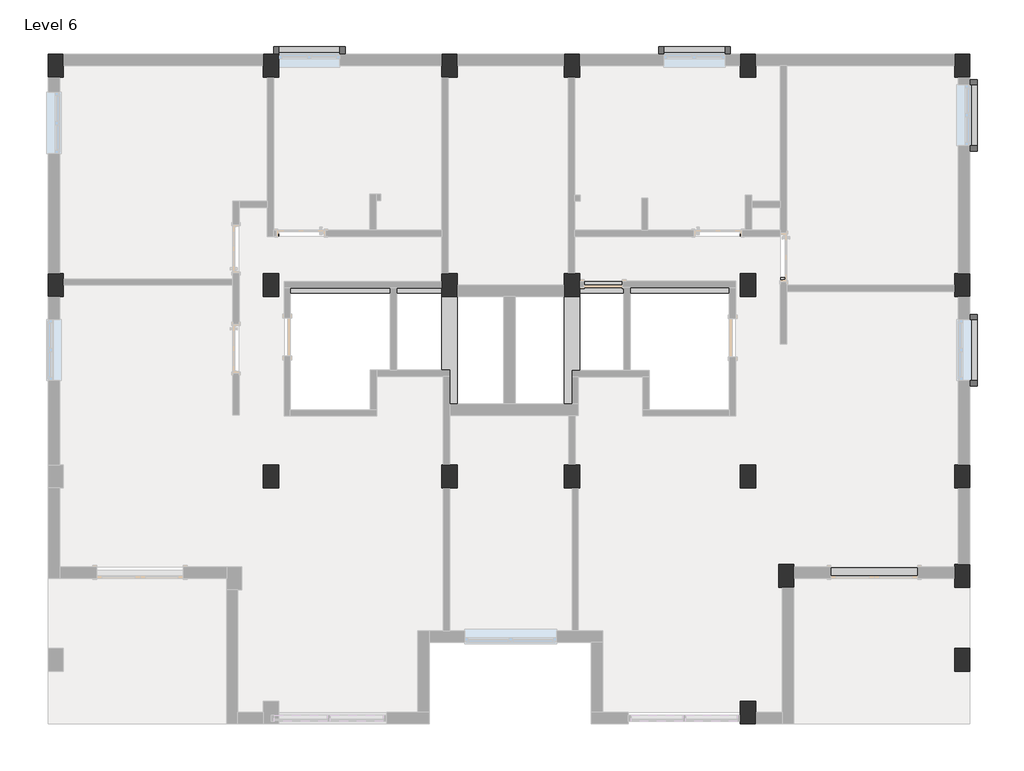
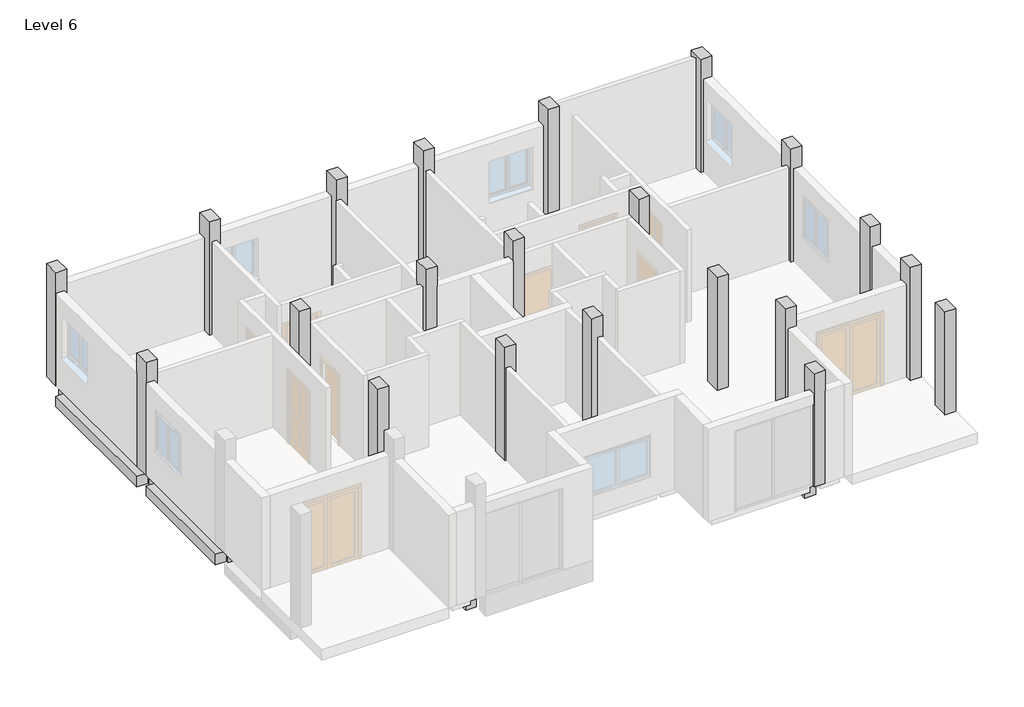
# One storey, part 3 of 3: 34 beams, 21 columns, 4 proxies.
"""IFC4 building model written with IfcOpenShell, lengths in millimetres."""

from ifc_helpers import new_model, si_unit, frame, origin, place, context, project, spatial, polyline, outline, extrude, faceted_brep, transform, mapped, element, save
from components import generic_models_13_generic_models_13_6edbfaa0, generic_models_10_generic_models_5_40bb8100, column_ab9bb308

model = new_model("IFC4")

# Units and contexts
model_context = context("Model", 3, world=origin())
ifc_project = project(units=[si_unit("LENGTHUNIT", "METRE", prefix="MILLI")], contexts=[model_context])

# Site, building, storey
site = spatial("IfcSite", under=ifc_project)
building = spatial("IfcBuilding", under=site)
storey = spatial("IfcBuildingStorey", under=building, Name="Level 6", Elevation=9448.8)

# Beams
placement = place(None, origin())
element("IfcBeam", 1, ObjectType="Concrete-Rectangular Beam : 12 x 24", at=placement, inside=storey, context=model_context, shape_type="SweptSolid", body=[
    extrude(outline(polyline([(-8839.9786397, -1604.6061634), (-8839.9786397, -1299.8061634), (-4852.9175798, -1299.8061634), (-4852.9175798, -1604.6061634), (-8839.9786397, -1604.6061634)])), frame((0.0, 0.0, 8839.2), z_axis=(0.0, 0.0, 1.0), x_axis=(1.0, 0.0, 0.0)), (0.0, 0.0, 1.0), 304.8),
])
element("IfcBeam", 2, ObjectType="Concrete-Rectangular Beam : 12 x 24", at=placement, inside=storey, context=model_context, shape_type="SweptSolid", body=[
    extrude(outline(polyline([(-1296.9175798, -1604.6061634), (-4548.1175798, -1604.6061634), (-4548.1175798, -1299.8061634), (-1296.9175798, -1299.8061634), (-1296.9175798, -1604.6061634)])), frame((0.0, 0.0, 8839.2), z_axis=(0.0, 0.0, 1.0), x_axis=(1.0, 0.0, 0.0)), (0.0, 0.0, 1.0), 304.8),
])
element("IfcBeam", 3, ObjectType="Concrete-Rectangular Beam : 12 x 24", at=placement, inside=storey, context=model_context, shape_type="SweptSolid", body=[
    extrude(outline(polyline([(1141.4824202, -1604.6061634), (-992.1175798, -1604.6061634), (-992.1175798, -1299.8061634), (1141.4824202, -1299.8061634), (1141.4824202, -1604.6061634)])), frame((0.0, 0.0, 8839.2), z_axis=(0.0, 0.0, 1.0), x_axis=(1.0, 0.0, 0.0)), (0.0, 0.0, 1.0), 304.8),
])
element("IfcBeam", 4, ObjectType="Concrete-Rectangular Beam : 12 x 24", at=placement, inside=storey, context=model_context, shape_type="SweptSolid", body=[
    extrude(outline(polyline([(4646.6824202, -1604.6061634), (1446.2824202, -1604.6061634), (1446.2824202, -1299.8061634), (4646.6824202, -1299.8061634), (4646.6824202, -1604.6061634)])), frame((0.0, 0.0, 8839.2), z_axis=(0.0, 0.0, 1.0), x_axis=(1.0, 0.0, 0.0)), (0.0, 0.0, 1.0), 304.8),
])
element("IfcBeam", 5, ObjectType="Concrete-Rectangular Beam : 12 x 24", at=placement, inside=storey, context=model_context, shape_type="SweptSolid", body=[
    extrude(outline(polyline([(8913.9345022, -1604.6061634), (4951.5345022, -1604.6061634), (4951.5345022, -1299.8061634), (8913.9345022, -1299.8061634), (8913.9345022, -1604.6061634)])), frame((0.0, 0.0, 8839.2), z_axis=(0.0, 0.0, 1.0), x_axis=(1.0, 0.0, 0.0)), (0.0, 0.0, 1.0), 304.8),
])
element("IfcBeam", 6, ObjectType="Concrete-Rectangular Beam : 12 x 24", at=placement, inside=storey, context=model_context, shape_type="SweptSolid", body=[
    extrude(outline(polyline([(8913.8824202, -5600.6620333), (8913.8824202, -1680.8061634), (9218.6824202, -1680.8061634), (9218.6824202, -5600.6620333), (8913.8824202, -5600.6620333)])), frame((0.0, 0.0, 8839.2), z_axis=(0.0, 0.0, 1.0), x_axis=(1.0, 0.0, 0.0)), (0.0, 0.0, 1.0), 304.8),
])
element("IfcBeam", 7, ObjectType="Concrete-Rectangular Beam : 12 x 24", at=placement, inside=storey, context=model_context, shape_type="SweptSolid", body=[
    extrude(outline(polyline([(8913.8824202, -9410.6620333), (8913.8824202, -6057.8620333), (9218.6824202, -6057.8620333), (9218.6824202, -9410.6620333), (8913.8824202, -9410.6620333)])), frame((0.0, 0.0, 8839.2), z_axis=(0.0, 0.0, 1.0), x_axis=(1.0, 0.0, 0.0)), (0.0, 0.0, 1.0), 304.8),
])
element("IfcBeam", 8, ObjectType="Concrete-Rectangular Beam : 12 x 24", at=placement, inside=storey, context=model_context, shape_type="SweptSolid", body=[
    extrude(outline(polyline([(8913.8824202, -11391.8620333), (8913.8824202, -9867.8620333), (9218.6824202, -9867.8620333), (9218.6824202, -11391.8620333), (8913.8824202, -11391.8620333)])), frame((0.0, 0.0, 8839.2), z_axis=(0.0, 0.0, 1.0), x_axis=(1.0, 0.0, 0.0)), (0.0, 0.0, 1.0), 304.8),
])
element("IfcBeam", 9, ObjectType="Concrete-Rectangular Beam : 12 x 24", at=placement, inside=storey, context=model_context, shape_type="SweptSolid", body=[
    extrude(outline(polyline([(-9144.7786397, -5600.6620333), (-9144.7786397, -1680.8061634), (-8839.9786397, -1680.8061634), (-8839.9786397, -5600.6620333), (-9144.7786397, -5600.6620333)])), frame((0.0, 0.0, 8839.2), z_axis=(0.0, 0.0, 1.0), x_axis=(1.0, 0.0, 0.0)), (0.0, 0.0, 1.0), 304.8),
])
element("IfcBeam", 10, ObjectType="Concrete-Rectangular Beam : 12 x 24", at=placement, inside=storey, context=model_context, shape_type="SweptSolid", body=[
    extrude(outline(polyline([(-9144.7786397, -9410.6620333), (-9144.7786397, -6057.8620333), (-8839.9786397, -6057.8620333), (-8839.9786397, -9410.6620333), (-9144.7786397, -9410.6620333)])), frame((0.0, 0.0, 8839.2), z_axis=(0.0, 0.0, 1.0), x_axis=(1.0, 0.0, 0.0)), (0.0, 0.0, 1.0), 304.8),
])
element("IfcBeam", 11, ObjectType="Concrete-Rectangular Beam : 12 x 24", at=placement, inside=storey, context=model_context, shape_type="SweptSolid", body=[
    extrude(outline(polyline([(4951.4824202, -5676.8620333), (8913.8824202, -5676.8620333), (8913.8824202, -5981.6620333), (4951.4824202, -5981.6620333), (4951.4824202, -5676.8620333)])), frame((0.0, 0.0, 8839.2), z_axis=(0.0, 0.0, 1.0), x_axis=(1.0, 0.0, 0.0)), (0.0, 0.0, 1.0), 304.8),
])
element("IfcBeam", 12, ObjectType="Concrete-Rectangular Beam : 12 x 24", at=placement, inside=storey, context=model_context, shape_type="SweptSolid", body=[
    extrude(outline(polyline([(1446.2824202, -5676.8620333), (4646.6824202, -5676.8620333), (4646.6824202, -5981.6620333), (1446.2824202, -5981.6620333), (1446.2824202, -5676.8620333)])), frame((0.0, 0.0, 8839.2), z_axis=(0.0, 0.0, 1.0), x_axis=(1.0, 0.0, 0.0)), (0.0, 0.0, 1.0), 304.8),
])
element("IfcBeam", 13, ObjectType="Concrete-Rectangular Beam : 12 x 24", at=placement, inside=storey, context=model_context, shape_type="SweptSolid", body=[
    extrude(outline(polyline([(-992.1175798, -5676.8620333), (1141.4824202, -5676.8620333), (1141.4824202, -5981.6620333), (-992.1175798, -5981.6620333), (-992.1175798, -5676.8620333)])), frame((0.0, 0.0, 8839.2), z_axis=(0.0, 0.0, 1.0), x_axis=(1.0, 0.0, 0.0)), (0.0, 0.0, 1.0), 304.8),
])
element("IfcBeam", 14, ObjectType="Concrete-Rectangular Beam : 12 x 24", at=placement, inside=storey, context=model_context, shape_type="SweptSolid", body=[
    extrude(outline(polyline([(-4548.1175798, -5676.8620333), (-1296.9175798, -5676.8620333), (-1296.9175798, -5981.6620333), (-4548.1175798, -5981.6620333), (-4548.1175798, -5676.8620333)])), frame((0.0, 0.0, 8839.2), z_axis=(0.0, 0.0, 1.0), x_axis=(1.0, 0.0, 0.0)), (0.0, 0.0, 1.0), 304.8),
])
element("IfcBeam", 15, ObjectType="Concrete-Rectangular Beam : 12 x 24", at=placement, inside=storey, context=model_context, shape_type="SweptSolid", body=[
    extrude(outline(polyline([(-8839.9786397, -5676.8620333), (-4852.9175798, -5676.8620333), (-4852.9175798, -5981.6620333), (-8839.9786397, -5981.6620333), (-8839.9786397, -5676.8620333)])), frame((0.0, 0.0, 8839.2), z_axis=(0.0, 0.0, 1.0), x_axis=(1.0, 0.0, 0.0)), (0.0, 0.0, 1.0), 304.8),
])
element("IfcBeam", 16, ObjectType="Concrete-Rectangular Beam : 12 x 24", at=placement, inside=storey, context=model_context, shape_type="SweptSolid", body=[
    extrude(outline(polyline([(-4852.9175798, -9791.6620333), (-8839.9786397, -9791.6620333), (-8839.9786397, -9486.8620333), (-4852.9175798, -9486.8620333), (-4852.9175798, -9791.6620333)])), frame((0.0, 0.0, 8839.2), z_axis=(0.0, 0.0, 1.0), x_axis=(1.0, 0.0, 0.0)), (0.0, 0.0, 1.0), 304.8),
])
element("IfcBeam", 17, ObjectType="Concrete-Rectangular Beam : 12 x 24", at=placement, inside=storey, context=model_context, shape_type="SweptSolid", body=[
    extrude(outline(polyline([(-1296.9175798, -9791.6620333), (-4548.1175798, -9791.6620333), (-4548.1175798, -9486.8620333), (-1296.9175798, -9486.8620333), (-1296.9175798, -9791.6620333)])), frame((0.0, 0.0, 8839.2), z_axis=(0.0, 0.0, 1.0), x_axis=(1.0, 0.0, 0.0)), (0.0, 0.0, 1.0), 304.8),
])
element("IfcBeam", 18, ObjectType="Concrete-Rectangular Beam : 12 x 24", at=placement, inside=storey, context=model_context, shape_type="SweptSolid", body=[
    extrude(outline(polyline([(1446.2824202, -9791.6620333), (1446.2824202, -9486.8620333), (4646.6824202, -9486.8620333), (4646.6824202, -9791.6620333), (1446.2824202, -9791.6620333)])), frame((0.0, 0.0, 8839.2), z_axis=(0.0, 0.0, 1.0), x_axis=(1.0, 0.0, 0.0)), (0.0, 0.0, 1.0), 304.8),
])
element("IfcBeam", 19, ObjectType="Concrete-Rectangular Beam : 12 x 24", at=placement, inside=storey, context=model_context, shape_type="Brep", body=[
    faceted_brep([(4646.6824202, -9867.8620333, 8839.2), (4646.6824202, -11772.8620333, 8839.2), (4646.6824202, -11772.8620333, 9144.0), (4646.6824202, -9867.8620333, 9144.0), (4951.4824202, -9867.8620333, 8839.2), (4951.4824202, -11468.0620333, 8839.2), (4951.4824202, -11772.8620333, 8839.2), (4951.4824202, -9867.8620333, 9144.0), (4951.4824202, -11468.0620333, 9144.0), (4951.4824202, -11772.8620333, 9144.0)], [[[0, 1, 2, 3]], [[1, 0, 4, 5, 6]], [[6, 5, 4, 7, 8, 9]], [[1, 6, 9, 2]], [[4, 0, 3, 7]], [[3, 2, 9, 8, 7]]]),
])
element("IfcBeam", 20, ObjectType="Concrete-Rectangular Beam : 12 x 24", at=placement, inside=storey, context=model_context, shape_type="SweptSolid", body=[
    extrude(outline(polyline([(4951.4824202, -11772.8620333), (4951.4824202, -11468.0620333), (5408.6824202, -11468.0620333), (5408.6824202, -11772.8620333), (4951.4824202, -11772.8620333)])), frame((0.0, 0.0, 8839.2), z_axis=(0.0, 0.0, 1.0), x_axis=(1.0, 0.0, 0.0)), (0.0, 0.0, 1.0), 304.8),
])
element("IfcBeam", 21, ObjectType="Concrete-Rectangular Beam : 12 x 24", at=placement, inside=storey, context=model_context, shape_type="SweptSolid", body=[
    extrude(outline(polyline([(8913.8824202, -11772.8620333), (5713.4824202, -11772.8620333), (5713.4824202, -11468.0620333), (8913.8824202, -11468.0620333), (8913.8824202, -11772.8620333)])), frame((0.0, 0.0, 8839.2), z_axis=(0.0, 0.0, 1.0), x_axis=(1.0, 0.0, 0.0)), (0.0, 0.0, 1.0), 304.8),
])
element("IfcBeam", 22, ObjectType="Concrete-Rectangular Beam : 12 x 24", at=placement, inside=storey, context=model_context, shape_type="Brep", body=[
    faceted_brep([(-4852.9175798, -9867.8620333, 8839.2), (-4852.9175798, -11518.8620333, 8839.2), (-4852.9175798, -11823.6620333, 8839.2), (-4852.9175798, -14119.6402089, 8839.2), (-4852.9175798, -14119.6402089, 9144.0), (-4852.9175798, -11823.6620333, 9144.0), (-4852.9175798, -11518.8620333, 9144.0), (-4852.9175798, -9867.8620333, 9144.0), (-4548.1175798, -9867.8620333, 8839.2), (-4548.1175798, -14119.6402089, 8839.2), (-4548.1175798, -9867.8620333, 9144.0), (-4548.1175798, -14119.6402089, 9144.0)], [[[0, 1, 2, 3, 4, 5, 6, 7]], [[3, 2, 1, 0, 8, 9]], [[9, 8, 10, 11]], [[8, 0, 7, 10]], [[3, 9, 11, 4]], [[7, 6, 5, 4, 11, 10]]]),
])
element("IfcBeam", 23, ObjectType="Concrete-Rectangular Beam : 12 x 24", at=placement, inside=storey, context=model_context, shape_type="SweptSolid", body=[
    extrude(outline(polyline([(-4852.9175798, -11823.6620333), (-5284.7175798, -11823.6620333), (-5284.7175798, -11518.8620333), (-4852.9175798, -11518.8620333), (-4852.9175798, -11823.6620333)])), frame((0.0, 0.0, 8839.2), z_axis=(0.0, 0.0, 1.0), x_axis=(1.0, 0.0, 0.0)), (0.0, 0.0, 1.0), 304.8),
])
element("IfcBeam", 24, ObjectType="Concrete-Rectangular Beam : 12 x 24", at=placement, inside=storey, context=model_context, shape_type="SweptSolid", body=[
    extrude(outline(polyline([(4951.4824202, -11772.8620333), (4951.4824202, -14119.6402089), (4646.6824202, -14119.6402089), (4646.6824202, -11772.8620333), (4951.4824202, -11772.8620333)])), frame((0.0, 0.0, 8839.2), z_axis=(0.0, 0.0, 1.0), x_axis=(1.0, 0.0, 0.0)), (0.0, 0.0, 1.0), 304.8),
])
element("IfcBeam", 25, ObjectType="Concrete-Rectangular Beam : 12 x 24", at=placement, inside=storey, context=model_context, shape_type="SweptSolid", body=[
    extrude(outline(polyline([(-4852.9175798, -5600.6620333), (-4852.9175798, -1680.8061634), (-4548.1175798, -1680.8061634), (-4548.1175798, -5600.6620333), (-4852.9175798, -5600.6620333)])), frame((0.0, 0.0, 8839.2), z_axis=(0.0, 0.0, 1.0), x_axis=(1.0, 0.0, 0.0)), (0.0, 0.0, 1.0), 304.8),
])
element("IfcBeam", 26, ObjectType="Concrete-Rectangular Beam : 12 x 24", at=placement, inside=storey, context=model_context, shape_type="SweptSolid", body=[
    extrude(outline(polyline([(-4852.9175798, -9410.6620333), (-4852.9175798, -6057.8620333), (-4548.1175798, -6057.8620333), (-4548.1175798, -9410.6620333), (-4852.9175798, -9410.6620333)])), frame((0.0, 0.0, 8839.2), z_axis=(0.0, 0.0, 1.0), x_axis=(1.0, 0.0, 0.0)), (0.0, 0.0, 1.0), 304.8),
])
element("IfcBeam", 27, ObjectType="Concrete-Rectangular Beam : 12 x 24", at=placement, inside=storey, context=model_context, shape_type="SweptSolid", body=[
    extrude(outline(polyline([(-1296.9175798, -5600.6620333), (-1296.9175798, -1680.8061634), (-992.1175798, -1680.8061634), (-992.1175798, -5600.6620333), (-1296.9175798, -5600.6620333)])), frame((0.0, 0.0, 8839.2), z_axis=(0.0, 0.0, 1.0), x_axis=(1.0, 0.0, 0.0)), (0.0, 0.0, 1.0), 304.8),
])
element("IfcBeam", 28, ObjectType="Concrete-Rectangular Beam : 12 x 24", at=placement, inside=storey, context=model_context, shape_type="SweptSolid", body=[
    extrude(outline(polyline([(-1296.9175798, -9410.6620333), (-1296.9175798, -6057.8620333), (-992.1175798, -6057.8620333), (-992.1175798, -9410.6620333), (-1296.9175798, -9410.6620333)])), frame((0.0, 0.0, 8839.2), z_axis=(0.0, 0.0, 1.0), x_axis=(1.0, 0.0, 0.0)), (0.0, 0.0, 1.0), 304.8),
])
element("IfcBeam", 29, ObjectType="Concrete-Rectangular Beam : 12 x 24", at=placement, inside=storey, context=model_context, shape_type="SweptSolid", body=[
    extrude(outline(polyline([(1446.2824202, -6057.8620333), (1446.2824202, -9410.6620333), (1141.4824202, -9410.6620333), (1141.4824202, -6057.8620333), (1446.2824202, -6057.8620333)])), frame((0.0, 0.0, 8839.2), z_axis=(0.0, 0.0, 1.0), x_axis=(1.0, 0.0, 0.0)), (0.0, 0.0, 1.0), 304.8),
])
element("IfcBeam", 30, ObjectType="Concrete-Rectangular Beam : 12 x 24", at=placement, inside=storey, context=model_context, shape_type="SweptSolid", body=[
    extrude(outline(polyline([(1446.2824202, -1680.8061634), (1446.2824202, -5600.6620333), (1141.4824202, -5600.6620333), (1141.4824202, -1680.8061634), (1446.2824202, -1680.8061634)])), frame((0.0, 0.0, 8839.2), z_axis=(0.0, 0.0, 1.0), x_axis=(1.0, 0.0, 0.0)), (0.0, 0.0, 1.0), 304.8),
])
element("IfcBeam", 31, ObjectType="Concrete-Rectangular Beam : 12 x 24", at=placement, inside=storey, context=model_context, shape_type="SweptSolid", body=[
    extrude(outline(polyline([(4646.6824202, -5600.6620333), (4646.6824202, -1680.8061634), (4951.4824202, -1680.8061634), (4951.4824202, -5600.6620333), (4646.6824202, -5600.6620333)])), frame((0.0, 0.0, 8839.2), z_axis=(0.0, 0.0, 1.0), x_axis=(1.0, 0.0, 0.0)), (0.0, 0.0, 1.0), 304.8),
])
element("IfcBeam", 32, ObjectType="Concrete-Rectangular Beam : 12 x 24", at=placement, inside=storey, context=model_context, shape_type="SweptSolid", body=[
    extrude(outline(polyline([(4646.6824202, -9410.6620333), (4646.6824202, -6057.8620333), (4951.4824202, -6057.8620333), (4951.4824202, -9410.6620333), (4646.6824202, -9410.6620333)])), frame((0.0, 0.0, 8839.2), z_axis=(0.0, 0.0, 1.0), x_axis=(1.0, 0.0, 0.0)), (0.0, 0.0, 1.0), 304.8),
])
element("IfcBeam", 33, ObjectType="Concrete-Rectangular Beam : 12 x 24", at=placement, inside=storey, context=model_context, shape_type="SweptSolid", body=[
    extrude(outline(polyline([(4951.4824202, -9486.8620333), (8913.8824202, -9486.8620333), (8913.8824202, -9791.6620333), (4951.4824202, -9791.6620333), (4951.4824202, -9486.8620333)])), frame((0.0, 0.0, 8839.2), z_axis=(0.0, 0.0, 1.0), x_axis=(1.0, 0.0, 0.0)), (0.0, 0.0, 1.0), 304.8),
])
element("IfcBeam", 34, ObjectType="Concrete-Rectangular Beam : 12 x 24", at=placement, inside=storey, context=model_context, shape_type="SweptSolid", body=[
    extrude(outline(polyline([(1141.4824202, -9486.8620333), (1141.4824202, -9791.6620333), (-992.1175798, -9791.6620333), (-992.1175798, -9486.8620333), (1141.4824202, -9486.8620333)])), frame((0.0, 0.0, 8839.2), z_axis=(0.0, 0.0, 1.0), x_axis=(1.0, 0.0, 0.0)), (0.0, 0.0, 1.0), 609.6),
])

# Proxies
generic_models_13_generic_models_13_shape = generic_models_13_generic_models_13_6edbfaa0(model_context)
element("IfcBuildingElementProxy", 35, Name="Generic Models 13 : Generic Models 13", ObjectType="Generic Models 13 : Generic Models 13", at=placement, inside=storey, context=model_context, shape_type="MappedRepresentation", body=[
    mapped(generic_models_13_generic_models_13_shape, transform((0.0, 0.0, 0.0), x_axis=(1.0, 0.0, 0.0), y_axis=(0.0, 1.0, 0.0), z_axis=(0.0, 0.0, 1.0))),
])
element("IfcBuildingElementProxy", 36, Name="Generic Models 14 : Generic Models 13", ObjectType="Generic Models 14 : Generic Models 13", at=placement, inside=storey, context=model_context, shape_type="MappedRepresentation", body=[
    mapped(generic_models_13_generic_models_13_shape, transform((-7670.8, 0.0, 0.0), x_axis=(1.0, 0.0, 0.0), y_axis=(0.0, 1.0, 0.0), z_axis=(0.0, 0.0, 1.0))),
])
generic_models_10_generic_models_5_shape = generic_models_10_generic_models_5_40bb8100(model_context)
element("IfcBuildingElementProxy", 37, Name="Generic Models 5 : Generic Models 5", ObjectType="Generic Models 5 : Generic Models 5", at=placement, inside=storey, context=model_context, shape_type="MappedRepresentation", body=[
    mapped(generic_models_10_generic_models_5_shape, transform((0.0, 0.0, 0.0), x_axis=(1.0, 0.0, 0.0), y_axis=(0.0, 1.0, 0.0), z_axis=(0.0, 0.0, 1.0))),
])
element("IfcBuildingElementProxy", 38, Name="Generic Models 6 : Generic Models 5", ObjectType="Generic Models 6 : Generic Models 5", at=placement, inside=storey, context=model_context, shape_type="MappedRepresentation", body=[
    mapped(generic_models_10_generic_models_5_shape, transform((0.0, 4681.8558699, 0.0), x_axis=(1.0, 0.0, 0.0), y_axis=(0.0, 1.0, 0.0), z_axis=(0.0, 0.0, 1.0))),
])

# Columns
element("IfcColumn", 39, ObjectType="Concrete-Rectangular-Column : 1'6\" X 1' COLUMN", at=placement, inside=storey, context=model_context, shape_type="Brep", body=[
    faceted_brep([(-8839.9786397, -1223.6061634, 9448.8), (-8839.9786397, -1680.8061634, 9448.8), (-9144.7786397, -1680.8061634, 9448.8), (-9144.7786397, -1223.6061634, 9448.8), (-8839.9786397, -1223.6061634, 12801.6), (-8839.9786397, -1680.8061634, 12801.6), (-8839.9786397, -1680.8061634, 9753.6), (-9144.7786397, -1680.8061634, 12801.6), (-9144.7786397, -1680.8061634, 9753.6), (-9144.7786397, -1223.6061634, 12801.6)], [[[0, 1, 2, 3]], [[4, 5, 6, 1, 0]], [[5, 7, 8, 2, 1, 6]], [[7, 9, 3, 2, 8]], [[9, 4, 0, 3]], [[4, 9, 7, 5]]]),
])
element("IfcColumn", 40, ObjectType="Concrete-Rectangular-Column : 1'6\" X 1' COLUMN", at=placement, inside=storey, context=model_context, shape_type="Brep", body=[
    faceted_brep([(-4548.1175798, -1223.6061634, 9448.8), (-4548.1175798, -1680.8061634, 9448.8), (-4852.9175798, -1680.8061634, 9448.8), (-4852.9175798, -1223.6061634, 9448.8), (-4548.1175798, -1223.6061634, 12801.6), (-4548.1175798, -1680.8061634, 12801.6), (-4548.1175798, -1680.8061634, 9753.6), (-4852.9175798, -1680.8061634, 12801.6), (-4852.9175798, -1680.8061634, 9753.6), (-4852.9175798, -1223.6061634, 12801.6)], [[[0, 1, 2, 3]], [[4, 5, 6, 1, 0]], [[5, 7, 8, 2, 1, 6]], [[7, 9, 3, 2, 8]], [[9, 4, 0, 3]], [[4, 9, 7, 5]]]),
])
element("IfcColumn", 41, ObjectType="Concrete-Rectangular-Column : 1'6\" X 1' COLUMN", at=placement, inside=storey, context=model_context, shape_type="Brep", body=[
    faceted_brep([(-992.1175798, -1223.6061634, 9448.8), (-992.1175798, -1680.8061634, 9448.8), (-1296.9175798, -1680.8061634, 9448.8), (-1296.9175798, -1223.6061634, 9448.8), (-992.1175798, -1223.6061634, 12801.6), (-992.1175798, -1680.8061634, 12801.6), (-992.1175798, -1680.8061634, 9753.6), (-1296.9175798, -1680.8061634, 12801.6), (-1296.9175798, -1680.8061634, 9753.6), (-1296.9175798, -1223.6061634, 12801.6)], [[[0, 1, 2, 3]], [[4, 5, 6, 1, 0]], [[5, 7, 8, 2, 1, 6]], [[7, 9, 3, 2, 8]], [[9, 4, 0, 3]], [[4, 9, 7, 5]]]),
])
element("IfcColumn", 42, ObjectType="Concrete-Rectangular-Column : 1'6\" X 1' COLUMN", at=placement, inside=storey, context=model_context, shape_type="Brep", body=[
    faceted_brep([(1446.2824202, -1223.6061634, 9448.8), (1446.2824202, -1680.8061634, 9448.8), (1141.4824202, -1680.8061634, 9448.8), (1141.4824202, -1223.6061634, 9448.8), (1446.2824202, -1223.6061634, 12801.6), (1446.2824202, -1680.8061634, 12801.6), (1446.2824202, -1680.8061634, 9753.6), (1141.4824202, -1680.8061634, 12801.6), (1141.4824202, -1680.8061634, 9753.6), (1141.4824202, -1223.6061634, 12801.6)], [[[0, 1, 2, 3]], [[4, 5, 6, 1, 0]], [[5, 7, 8, 2, 1, 6]], [[7, 9, 3, 2, 8]], [[9, 4, 0, 3]], [[4, 9, 7, 5]]]),
])
element("IfcColumn", 43, ObjectType="Concrete-Rectangular-Column : 1'6\" X 1' COLUMN", at=placement, inside=storey, context=model_context, shape_type="Brep", body=[
    faceted_brep([(4951.4824202, -1223.6061634, 9448.8), (4951.4824202, -1680.8061634, 9448.8), (4646.6824202, -1680.8061634, 9448.8), (4646.6824202, -1223.6061634, 9448.8), (4951.4824202, -1223.6061634, 12801.6), (4951.4824202, -1680.8061634, 12801.6), (4951.4824202, -1680.8061634, 9753.6), (4646.6824202, -1680.8061634, 12801.6), (4646.6824202, -1680.8061634, 9753.6), (4646.6824202, -1223.6061634, 12801.6)], [[[0, 1, 2, 3]], [[4, 5, 6, 1, 0]], [[5, 7, 8, 2, 1, 6]], [[7, 9, 3, 2, 8]], [[9, 4, 0, 3]], [[4, 9, 7, 5]]]),
])
element("IfcColumn", 44, ObjectType="Concrete-Rectangular-Column : 1'6\" X 1' COLUMN", at=placement, inside=storey, context=model_context, shape_type="Brep", body=[
    faceted_brep([(9218.6824202, -1223.6061634, 9448.8), (9218.6824202, -1680.8061634, 9448.8), (8913.8824202, -1680.8061634, 9448.8), (8913.8824202, -1223.6061634, 9448.8), (9218.6824202, -1223.6061634, 12801.6), (9218.6824202, -1680.8061634, 12801.6), (9218.6824202, -1680.8061634, 9753.6), (8913.8824202, -1680.8061634, 12801.6), (8913.8824202, -1680.8061634, 9753.6), (8913.8824202, -1223.6061634, 12801.6)], [[[0, 1, 2, 3]], [[4, 5, 6, 1, 0]], [[5, 7, 8, 2, 1, 6]], [[7, 9, 3, 2, 8]], [[9, 4, 0, 3]], [[4, 9, 7, 5]]]),
])
element("IfcColumn", 45, ObjectType="Concrete-Rectangular-Column : 1'6\" X 1' COLUMN", at=placement, inside=storey, context=model_context, shape_type="Brep", body=[
    faceted_brep([(9218.6824202, -5600.6620333, 9448.8), (9218.6824202, -6057.8620333, 9448.8), (8913.8824202, -6057.8620333, 9448.8), (8913.8824202, -5600.6620333, 9448.8), (9218.6824202, -5600.6620333, 12801.6), (9218.6824202, -6057.8620333, 12801.6), (9218.6824202, -6057.8620333, 9753.6), (9218.6824202, -5600.6620333, 9753.6), (8913.8824202, -6057.8620333, 12801.6), (8913.8824202, -6057.8620333, 9753.6), (8913.8824202, -5600.6620333, 12801.6), (8913.8824202, -5600.6620333, 9753.6)], [[[0, 1, 2, 3]], [[4, 5, 6, 1, 0, 7]], [[5, 8, 9, 2, 1, 6]], [[8, 10, 11, 3, 2, 9]], [[10, 4, 7, 0, 3, 11]], [[4, 10, 8, 5]]]),
])
element("IfcColumn", 46, ObjectType="Concrete-Rectangular-Column : 1'6\" X 1' COLUMN", at=placement, inside=storey, context=model_context, shape_type="Brep", body=[
    faceted_brep([(4951.4824202, -5600.6620333, 9448.8), (4951.4824202, -6057.8620333, 9448.8), (4646.6824202, -6057.8620333, 9448.8), (4646.6824202, -5600.6620333, 9448.8), (4951.4824202, -5600.6620333, 12801.6), (4951.4824202, -6057.8620333, 12801.6), (4951.4824202, -6057.8620333, 9753.6), (4951.4824202, -5600.6620333, 9753.6), (4646.6824202, -6057.8620333, 12801.6), (4646.6824202, -6057.8620333, 9753.6), (4646.6824202, -5600.6620333, 12801.6), (4646.6824202, -5600.6620333, 9753.6)], [[[0, 1, 2, 3]], [[4, 5, 6, 1, 0, 7]], [[5, 8, 9, 2, 1, 6]], [[8, 10, 11, 3, 2, 9]], [[10, 4, 7, 0, 3, 11]], [[4, 10, 8, 5]]]),
])
element("IfcColumn", 47, ObjectType="Concrete-Rectangular-Column : 1'6\" X 1' COLUMN", at=placement, inside=storey, context=model_context, shape_type="Brep", body=[
    faceted_brep([(1446.2824202, -5600.6620333, 9448.8), (1446.2824202, -6057.8620333, 9448.8), (1141.4824202, -6057.8620333, 9448.8), (1141.4824202, -5600.6620333, 9448.8), (1446.2824202, -5600.6620333, 12801.6), (1446.2824202, -6057.8620333, 12801.6), (1446.2824202, -6057.8620333, 9753.6), (1446.2824202, -5600.6620333, 9753.6), (1141.4824202, -6057.8620333, 12801.6), (1141.4824202, -6057.8620333, 9753.6), (1141.4824202, -5600.6620333, 12801.6), (1141.4824202, -5600.6620333, 9753.6)], [[[0, 1, 2, 3]], [[4, 5, 6, 1, 0, 7]], [[5, 8, 9, 2, 1, 6]], [[8, 10, 11, 3, 2, 9]], [[10, 4, 7, 0, 3, 11]], [[4, 10, 8, 5]]]),
])
element("IfcColumn", 48, ObjectType="Concrete-Rectangular-Column : 1'6\" X 1' COLUMN", at=placement, inside=storey, context=model_context, shape_type="Brep", body=[
    faceted_brep([(-992.1175798, -5600.6620333, 9448.8), (-992.1175798, -6057.8620333, 9448.8), (-1296.9175798, -6057.8620333, 9448.8), (-1296.9175798, -5600.6620333, 9448.8), (-992.1175798, -5600.6620333, 12801.6), (-992.1175798, -6057.8620333, 12801.6), (-992.1175798, -6057.8620333, 9753.6), (-992.1175798, -5600.6620333, 9753.6), (-1296.9175798, -6057.8620333, 12801.6), (-1296.9175798, -6057.8620333, 9753.6), (-1296.9175798, -5600.6620333, 12801.6), (-1296.9175798, -5600.6620333, 9753.6)], [[[0, 1, 2, 3]], [[4, 5, 6, 1, 0, 7]], [[5, 8, 9, 2, 1, 6]], [[8, 10, 11, 3, 2, 9]], [[10, 4, 7, 0, 3, 11]], [[4, 10, 8, 5]]]),
])
element("IfcColumn", 49, ObjectType="Concrete-Rectangular-Column : 1'6\" X 1' COLUMN", at=placement, inside=storey, context=model_context, shape_type="Brep", body=[
    faceted_brep([(-4548.1175798, -5600.6620333, 9448.8), (-4548.1175798, -6057.8620333, 9448.8), (-4852.9175798, -6057.8620333, 9448.8), (-4852.9175798, -5600.6620333, 9448.8), (-4548.1175798, -5600.6620333, 12801.6), (-4548.1175798, -6057.8620333, 12801.6), (-4548.1175798, -6057.8620333, 9753.6), (-4548.1175798, -5600.6620333, 9753.6), (-4852.9175798, -6057.8620333, 12801.6), (-4852.9175798, -6057.8620333, 9753.6), (-4852.9175798, -5600.6620333, 12801.6), (-4852.9175798, -5600.6620333, 9753.6)], [[[0, 1, 2, 3]], [[4, 5, 6, 1, 0, 7]], [[5, 8, 9, 2, 1, 6]], [[8, 10, 11, 3, 2, 9]], [[10, 4, 7, 0, 3, 11]], [[4, 10, 8, 5]]]),
])
element("IfcColumn", 50, ObjectType="Concrete-Rectangular-Column : 1'6\" X 1' COLUMN", at=placement, inside=storey, context=model_context, shape_type="Brep", body=[
    faceted_brep([(-8839.9786397, -5600.6620333, 9448.8), (-8839.9786397, -6057.8620333, 9448.8), (-9144.7786397, -6057.8620333, 9448.8), (-9144.7786397, -5600.6620333, 9448.8), (-8839.9786397, -5600.6620333, 12801.6), (-8839.9786397, -6057.8620333, 12801.6), (-8839.9786397, -6057.8620333, 9753.6), (-8839.9786397, -5600.6620333, 9753.6), (-9144.7786397, -6057.8620333, 12801.6), (-9144.7786397, -6057.8620333, 9753.6), (-9144.7786397, -5600.6620333, 12801.6), (-9144.7786397, -5600.6620333, 9753.6)], [[[0, 1, 2, 3]], [[4, 5, 6, 1, 0, 7]], [[5, 8, 9, 2, 1, 6]], [[8, 10, 11, 3, 2, 9]], [[10, 4, 7, 0, 3, 11]], [[4, 10, 8, 5]]]),
])
element("IfcColumn", 51, ObjectType="Concrete-Rectangular-Column : 1'6\" X 1' COLUMN", at=placement, inside=storey, context=model_context, shape_type="Brep", body=[
    faceted_brep([(-4548.1175798, -9410.6620333, 9448.8), (-4548.1175798, -9867.8620333, 9448.8), (-4852.9175798, -9867.8620333, 9448.8), (-4852.9175798, -9410.6620333, 9448.8), (-4548.1175798, -9410.6620333, 12801.6), (-4548.1175798, -9867.8620333, 12801.6), (-4548.1175798, -9867.8620333, 9753.6), (-4548.1175798, -9410.6620333, 9753.6), (-4852.9175798, -9867.8620333, 12801.6), (-4852.9175798, -9867.8620333, 9753.6), (-4852.9175798, -9410.6620333, 12801.6), (-4852.9175798, -9410.6620333, 9753.6)], [[[0, 1, 2, 3]], [[4, 5, 6, 1, 0, 7]], [[5, 8, 9, 2, 1, 6]], [[8, 10, 11, 3, 2, 9]], [[10, 4, 7, 0, 3, 11]], [[4, 10, 8, 5]]]),
])
element("IfcColumn", 52, ObjectType="Concrete-Rectangular-Column : 1'6\" X 1' COLUMN", at=placement, inside=storey, context=model_context, shape_type="Brep", body=[
    faceted_brep([(-992.1175798, -9410.6620333, 9448.8), (-992.1175798, -9867.8620333, 9448.8), (-1296.9175798, -9867.8620333, 9448.8), (-1296.9175798, -9410.6620333, 9448.8), (-992.1175798, -9410.6620333, 12801.6), (-992.1175798, -9867.8620333, 12801.6), (-992.1175798, -9410.6620333, 9753.6), (-1296.9175798, -9867.8620333, 12801.6), (-1296.9175798, -9410.6620333, 12801.6), (-1296.9175798, -9410.6620333, 9753.6)], [[[0, 1, 2, 3]], [[4, 5, 1, 0, 6]], [[5, 7, 2, 1]], [[7, 8, 9, 3, 2]], [[8, 4, 6, 0, 3, 9]], [[4, 8, 7, 5]]]),
])
element("IfcColumn", 53, ObjectType="Concrete-Rectangular-Column : 1'6\" X 1' COLUMN", at=placement, inside=storey, context=model_context, shape_type="Brep", body=[
    faceted_brep([(9218.6824202, -11391.8620333, 9448.8), (9218.6824202, -11849.0620333, 9448.8), (8913.8824202, -11849.0620333, 9448.8), (8913.8824202, -11391.8620333, 9448.8), (9218.6824202, -11391.8620333, 12801.6), (9218.6824202, -11849.0620333, 12801.6), (9218.6824202, -11391.8620333, 9753.6), (8913.8824202, -11849.0620333, 12801.6), (8913.8824202, -11391.8620333, 12801.6), (8913.8824202, -11391.8620333, 9753.6)], [[[0, 1, 2, 3]], [[4, 5, 1, 0, 6]], [[5, 7, 2, 1]], [[7, 8, 9, 3, 2]], [[8, 4, 6, 0, 3, 9]], [[4, 8, 7, 5]]]),
])
element("IfcColumn", 54, ObjectType="Concrete-Rectangular-Column : 1'6\" X 1' COLUMN", at=placement, inside=storey, context=model_context, shape_type="Brep", body=[
    faceted_brep([(9218.6824202, -9410.6620333, 9448.8), (9218.6824202, -9867.8620333, 9448.8), (8913.8824202, -9867.8620333, 9448.8), (8913.8824202, -9410.6620333, 9448.8), (9218.6824202, -9410.6620333, 12801.6), (9218.6824202, -9867.8620333, 12801.6), (9218.6824202, -9867.8620333, 9753.6), (9218.6824202, -9410.6620333, 9753.6), (8913.8824202, -9867.8620333, 12801.6), (8913.8824202, -9867.8620333, 9753.6), (8913.8824202, -9410.6620333, 12801.6), (8913.8824202, -9410.6620333, 9753.6)], [[[0, 1, 2, 3]], [[4, 5, 6, 1, 0, 7]], [[5, 8, 9, 2, 1, 6]], [[8, 10, 11, 3, 2, 9]], [[10, 4, 7, 0, 3, 11]], [[4, 10, 8, 5]]]),
])
element("IfcColumn", 55, ObjectType="Concrete-Rectangular-Column : 1'6\" X 1' COLUMN", at=placement, inside=storey, context=model_context, shape_type="Brep", body=[
    faceted_brep([(4951.4824202, -9410.6620333, 9448.8), (4951.4824202, -9867.8620333, 9448.8), (4646.6824202, -9867.8620333, 9448.8), (4646.6824202, -9410.6620333, 9448.8), (4951.4824202, -9410.6620333, 12801.6), (4951.4824202, -9867.8620333, 12801.6), (4951.4824202, -9867.8620333, 9753.6), (4951.4824202, -9410.6620333, 9753.6), (4646.6824202, -9867.8620333, 12801.6), (4646.6824202, -9867.8620333, 9753.6), (4646.6824202, -9410.6620333, 12801.6), (4646.6824202, -9410.6620333, 9753.6)], [[[0, 1, 2, 3]], [[4, 5, 6, 1, 0, 7]], [[5, 8, 9, 2, 1, 6]], [[8, 10, 11, 3, 2, 9]], [[10, 4, 7, 0, 3, 11]], [[4, 10, 8, 5]]]),
])
element("IfcColumn", 56, ObjectType="Concrete-Rectangular-Column : 1'6\" X 1' COLUMN", at=placement, inside=storey, context=model_context, shape_type="Brep", body=[
    faceted_brep([(1446.2824202, -9410.6620333, 9448.8), (1446.2824202, -9867.8620333, 9448.8), (1141.4824202, -9867.8620333, 9448.8), (1141.4824202, -9410.6620333, 9448.8), (1446.2824202, -9410.6620333, 12801.6), (1446.2824202, -9867.8620333, 12801.6), (1446.2824202, -9410.6620333, 9753.6), (1141.4824202, -9867.8620333, 12801.6), (1141.4824202, -9410.6620333, 12801.6), (1141.4824202, -9410.6620333, 9753.6)], [[[0, 1, 2, 3]], [[4, 5, 1, 0, 6]], [[5, 7, 2, 1]], [[7, 8, 9, 3, 2]], [[8, 4, 6, 0, 3, 9]], [[4, 8, 7, 5]]]),
])
element("IfcColumn", 57, ObjectType="Concrete-Rectangular-Column : 1'6\" X 1' COLUMN", at=placement, inside=storey, context=model_context, shape_type="SweptSolid", body=[
    extrude(outline(polyline([(5713.4824202, -11391.8620333), (5713.4824202, -11849.0620333), (5408.6824202, -11849.0620333), (5408.6824202, -11391.8620333), (5713.4824202, -11391.8620333)])), frame((0.0, 0.0, 9448.8), z_axis=(0.0, 0.0, 1.0), x_axis=(1.0, 0.0, 0.0)), (0.0, 0.0, 1.0), 3352.8),
])
element("IfcColumn", 58, ObjectType="Concrete-Rectangular-Column : 1'6\" X 1' COLUMN", at=placement, inside=storey, context=model_context, shape_type="Brep", body=[
    faceted_brep([(4951.4824202, -14119.6402089, 9448.8), (4951.4824202, -14576.8402089, 9448.8), (4646.6824202, -14576.8402089, 9448.8), (4646.6824202, -14119.6402089, 9448.8), (4951.4824202, -14119.6402089, 12801.6), (4951.4824202, -14576.8402089, 12801.6), (4951.4824202, -14119.6402089, 9753.6), (4646.6824202, -14576.8402089, 12801.6), (4646.6824202, -14119.6402089, 12801.6), (4646.6824202, -14119.6402089, 9753.6)], [[[0, 1, 2, 3]], [[4, 5, 1, 0, 6]], [[5, 7, 2, 1]], [[7, 8, 9, 3, 2]], [[8, 4, 6, 0, 3, 9]], [[4, 8, 7, 5]]]),
])
column_shape = column_ab9bb308(model_context)
element("IfcColumn", 59, ObjectType="Concrete-Rectangular-Column : 1'6\" X 1' COLUMN", at=placement, inside=storey, context=model_context, shape_type="MappedRepresentation", body=[
    mapped(column_shape, transform((9066.2824202, -13294.1402089, 0.0), x_axis=(1.0, 0.0, 0.0), y_axis=(0.0, 1.0, 0.0), z_axis=(0.0, 0.0, 1.0))),
])

save(model, "model.ifc")

# Revit data of these elements
# Type "Concrete-Rectangular Beam : 12 x 24"
#   Assembly Code = "B10"
#   Length [instance default] = 5' - 0"
#   b = 1' - 0"
#   h = 2' - 0"
#   Structural Material [instance default] = Concrete, Cast-in-Place gray
# Type "Concrete-Rectangular-Column : 1'6\" X 1' COLUMN"
#   Assembly Code = "B10"
#   b = 1' - 0"
#   h = 1' - 6"
#   Structural Material [instance default] = Concrete, Cast-in-Place gray
# Elements 1, 2, 3, 4, 5, 6, 7, 9, 10, 11, 12, 13, 14, 15, 16, 17, 18, 19, 20, 21, 22, 23, 24, 25, 26, 27, 28, 29, 30, 31, 32, 33, 34 (IfcBeam, "Concrete-Rectangular Beam : 12 x 24")
#   Structural Material = WARM BEIGE COLOUR
#   Phase Created = New Construction
#   Materials on its faces: "WARM BEIGE COLOUR"
# Element 8 (IfcBeam, "Concrete-Rectangular Beam : 12 x 24")
#   Length = 5' - 0"
#   Structural Material = WARM BEIGE COLOUR
#   Phase Created = New Construction
#   Materials on its faces: "WARM BEIGE COLOUR"
# Element 35 (IfcBuildingElementProxy, "Generic Models 13 : Generic Models 13")
#   Phase Created = New Construction
#   Materials on its faces: "black accent wall"
# Element 36 (IfcBuildingElementProxy, "Generic Models 14 : Generic Models 13")
#   Phase Created = New Construction
#   Materials on its faces: "black accent wall"
# Element 37 (IfcBuildingElementProxy, "Generic Models 5 : Generic Models 5")
#   Phase Created = New Construction
#   Materials on its faces: "black accent wall"
# Element 38 (IfcBuildingElementProxy, "Generic Models 6 : Generic Models 5")
#   Phase Created = New Construction
#   Materials on its faces: "black accent wall"
# Elements 39, 40, 41, 42, 43, 44, 45, 46, 47, 48, 49, 50, 51, 52, 53, 54, 55, 56, 57, 58, 59 (IfcColumn, "Concrete-Rectangular-Column : 1'6\" X 1' COLUMN")
#   Structural Material = WARM BEIGE COLOUR
#   Phase Created = New Construction
#   Materials on its faces: "WARM BEIGE COLOUR"
# Materials
#   "Concrete, Cast-in-Place gray": class "Concrete", colour RGB 192 192 192, transparency 0, Description = "Cast-in-place concrete", Cost = 0
#   "WARM BEIGE COLOUR": class "Generic", colour RGB 120 120 120, transparency 0, Cost = 0
#   "black accent wall": class "Generic", colour RGB 120 120 120, transparency 0, Cost = 0
